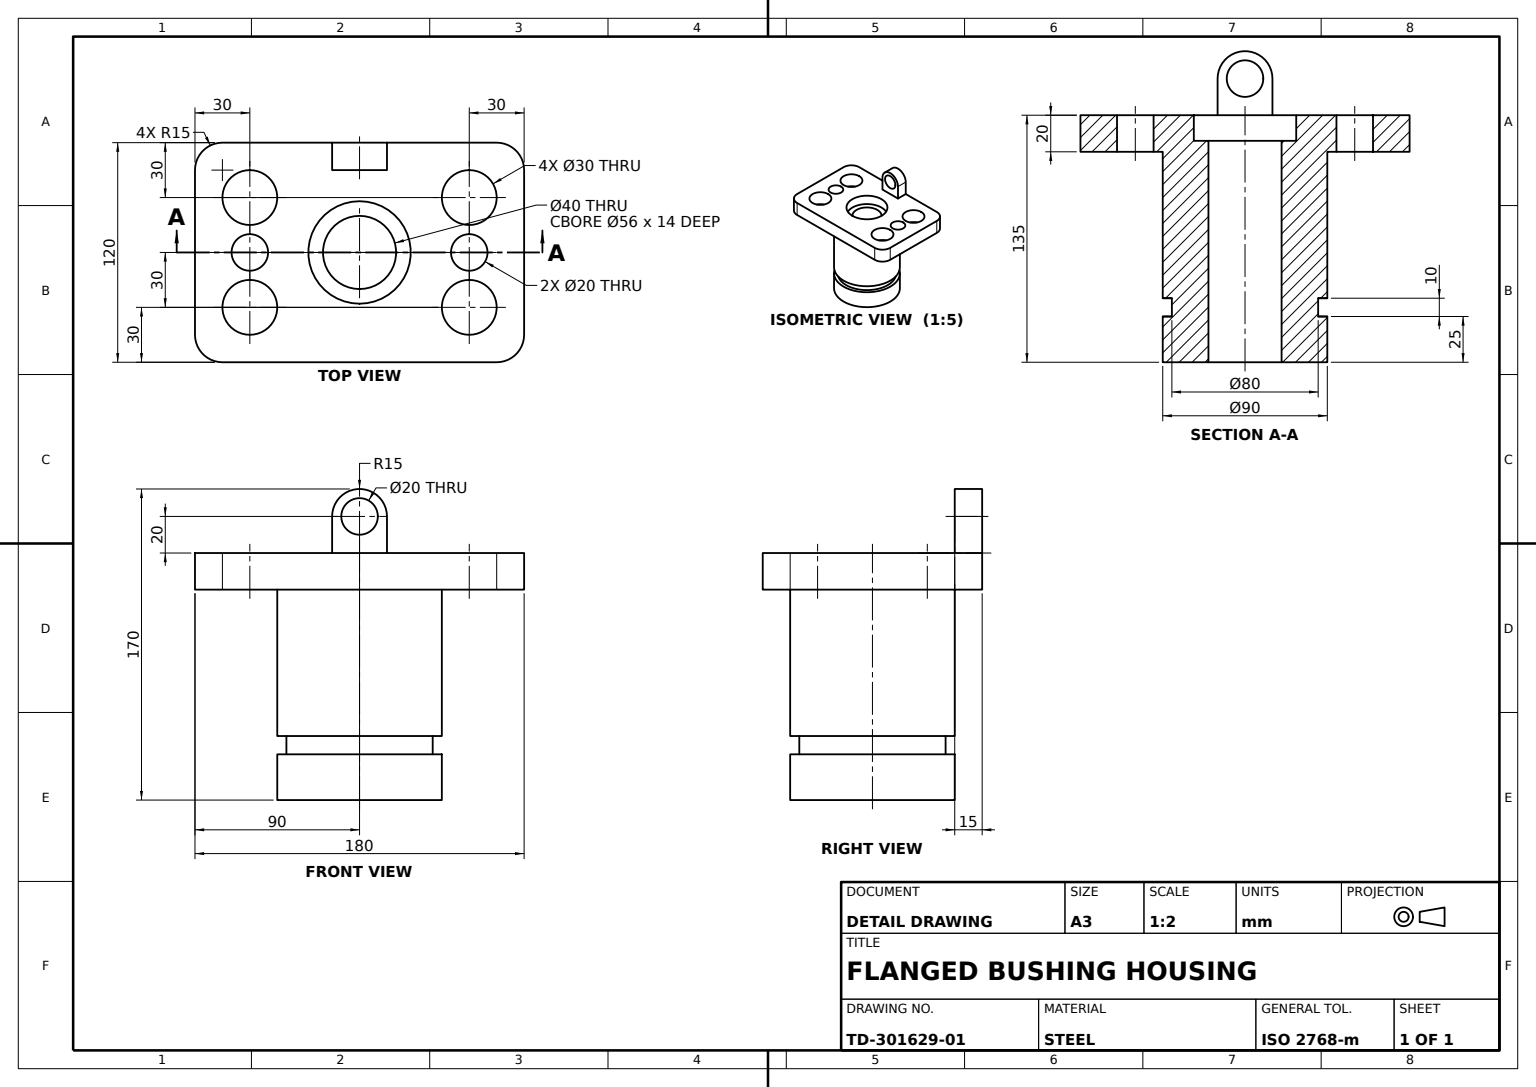
from build123d import *

# Parameters (mm, degrees)
FLANGE_START               = -20
FLANGE_PLATE_SKETCH_R      = 15
FLANGE_PLATE_SKETCH_R_2    = 10
FLANGE_PLATE_SKETCH_R_3    = 45
FLANGE_PLATE_120X180_DEPTH = 20
EYELET_LUG_SKETCH_R        = 10
EYELET_LUG_DEPTH           = 15


with BuildPart() as part:
    # Bushing Profile Sketch → Bushing Body (revolve)
    with BuildSketch(Plane.XY, mode=Mode.PRIVATE) as bushing_body_sk:
        Polygon((45, 0), (45, -100), (40, -100), (40, -110), (45, -110), (45, -135), (20, -135), (20, -14), (28, -14), (28, 0), align=None)
    revolve(bushing_body_sk.sketch.rotate(Axis((0, -88.636319954, 0), (0, 1, 0)), 90), axis=Axis((0, -88.636319954, 0), (0, 1, 0)))

    # Flange Plate Sketch → Flange Plate 120x180 (add)
    with BuildSketch(Plane(origin=(0, 0, 0), x_dir=(1, 0, 0), z_dir=(0, 1, 0)).offset(FLANGE_START)):
        with BuildLine():
            Line((-75, -60), (75, -60))
            ThreePointArc((75, -60), (85.606601718, -55.606601718), (90, -45))
            Line((90, -45), (90, 45))
            ThreePointArc((90, 45), (85.606601718, 55.606601718), (75, 60))
            Line((75, 60), (-75, 60))
            ThreePointArc((-75, 60), (-85.606601718, 55.606601718), (-90, 45))
            Line((-90, 45), (-90, -45))
            ThreePointArc((-90, -45), (-85.606601718, -55.606601718), (-75, -60))
        make_face()
        with Locations(Location((-60, -30, 0), (0, 0, 270))):
            Circle(FLANGE_PLATE_SKETCH_R, mode=Mode.SUBTRACT)
        with Locations(Location((-60, 0, 0), (0, 0, 270))):
            Circle(FLANGE_PLATE_SKETCH_R_2, mode=Mode.SUBTRACT)
        with Locations(Location((-60, 30, 0), (0, 0, 270))):
            Circle(FLANGE_PLATE_SKETCH_R, mode=Mode.SUBTRACT)
        with Locations(Location((60, -30, 0), (0, 0, 90))):
            Circle(FLANGE_PLATE_SKETCH_R, mode=Mode.SUBTRACT)
        with Locations(Location((60, 0, 0), (0, 0, 90))):
            Circle(FLANGE_PLATE_SKETCH_R_2, mode=Mode.SUBTRACT)
        with Locations(Location((60, 30, 0), (0, 0, 90))):
            Circle(FLANGE_PLATE_SKETCH_R, mode=Mode.SUBTRACT)
        with Locations(Location((0, 0, 0), (0, 0, 90))):
            Circle(FLANGE_PLATE_SKETCH_R_3, mode=Mode.SUBTRACT)
    extrude(amount=FLANGE_PLATE_120X180_DEPTH)

    # Eyelet Lug Sketch → Eyelet Lug (add)
    with BuildSketch(Plane(origin=(0, 0, -60), x_dir=(-1, 0, 0), z_dir=(0, 0, -1))):
        with BuildLine():
            Line((-15, 20), (-15, 0))
            Line((-15, 0), (15, 0))
            Line((15, 0), (15, 20))
            ThreePointArc((15, 20), (0, 35), (-15, 20))
        make_face()
        with Locations((0, 20)):
            Circle(EYELET_LUG_SKETCH_R, mode=Mode.SUBTRACT)
    extrude(amount=-EYELET_LUG_DEPTH)


solid = part.part
